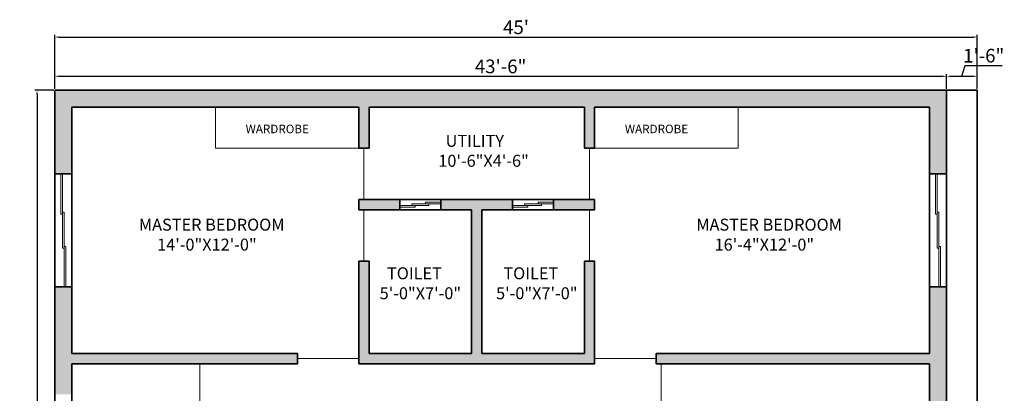
# Model space of a CAD drawing. Units: inches. Extents: x 3491 to 6898, y 1360 to 2019.
# Tile 3 of 9: x 3512 to 4088, y 1795 to 2013. Entities that reach past the tile are written whole.
import ezdxf

# ---------------------------------------------------------------- set-up
doc = ezdxf.new("R2010")
doc.units = ezdxf.units.IN
for name, color, linetype, lineweight in [('A-ANNO-DIMS', 2, 'Continuous', 18), ('A-ANNO-TEXT', 7, 'Continuous', 18), ('A-AREA-IDEN', 7, 'Continuous', 18), ('A-DOOR', 4, 'Continuous', 18), ('A-FLOR-CASE', 8, 'Continuous', 18), ('A-GLAZ', 5, 'Continuous', 18), ('A-WALL', 7, 'Continuous', 35), ('A-WALL-PATT', 8, 'Continuous', 13)]:
    doc.layers.add(name, color=color, linetype=linetype, lineweight=lineweight)
doc.styles.get("Standard").update_dxf_attribs({"font": 'arial.ttf'})
doc.dimstyles.new('ISO-25', dxfattribs={"dimtxt": 8, "dimasz": 2.5, "dimexe": 1.25, "dimexo": 0.625, "dimtad": 1, "dimdec": 1, "dimlunit": 3, "dimtxsty": 'Standard', "dimcen": 2.5, "dimclrt": 1, "dimadec": 0, "dimazin": 0, "dimtfac": 1, "dimtdec": 1, "dimtmove": 0, "dimatfit": 3, "dimfxl": 1, "dimarcsym": 0})

# ---------------------------------------------------------------- blocks, each defined once
blk = doc.blocks.new('*D1')
at = {"layer": 'A-ANNO-DIMS', "color": 0, "lineweight": -2, "transparency": 16777216}
for p, q in [((3532.13, 1972.99), (3532.13, 1981.69)), ((3534.63, 1980.44), (4051.63, 1980.44)), ((4054.13, 1972.99), (4054.13, 1981.69))]:
    blk.add_line(p, q, dxfattribs=at)
at = {"layer": 'A-ANNO-DIMS', "color": 0, "transparency": 16777216}
for points in [[(3534.63, 1980.85), (3534.63, 1980.02), (3532.13, 1980.44)], [(4051.63, 1980.85), (4051.63, 1980.02), (4054.13, 1980.44)]]:
    blk.add_solid(points, dxfattribs=at)
at = {"layer": 'Defpoints', "color": 0, "transparency": 16777216}
for p in [(4054.13, 1980.44), (3532.13, 1972.37), (4054.13, 1972.37)]:
    blk.add_point(p, dxfattribs=at)
at = {"layer": 'A-ANNO-DIMS', "color": 0, "transparency": 16777216, "insert": (3793.13, 1985.15), "char_height": 8, "attachment_point": 5}
blk.add_mtext('43\'-6"', dxfattribs=at)
blk = doc.blocks.new('*D2')
at = {"layer": 'A-ANNO-DIMS', "color": 0, "lineweight": -2, "transparency": 16777216}
for p, q in [((4063.13, 1980.44), (4065.01, 1986.71)), ((4065.01, 1986.71), (4086.78, 1986.71)), ((4054.13, 1972.99), (4054.13, 1981.69)), ((4056.63, 1980.44), (4069.63, 1980.44)), ((4072.13, 1972.99), (4072.13, 1981.69))]:
    blk.add_line(p, q, dxfattribs=at)
at = {"layer": 'A-ANNO-DIMS', "color": 0, "transparency": 16777216}
for points in [[(4056.63, 1980.85), (4056.63, 1980.02), (4054.13, 1980.44)], [(4069.63, 1980.85), (4069.63, 1980.02), (4072.13, 1980.44)]]:
    blk.add_solid(points, dxfattribs=at)
at = {"layer": 'Defpoints', "color": 0, "transparency": 16777216}
for p in [(4072.13, 1980.44), (4054.13, 1972.37), (4072.13, 1972.37)]:
    blk.add_point(p, dxfattribs=at)
at = {"layer": 'A-ANNO-DIMS', "color": 0, "transparency": 16777216, "insert": (4075.9, 1991.42), "char_height": 8, "attachment_point": 5}
blk.add_mtext('1\'-6"', dxfattribs=at)
blk = doc.blocks.new('*D3')
at = {"layer": 'A-ANNO-DIMS', "color": 0, "lineweight": -2, "transparency": 16777216}
for p, q in [((3532.13, 1972.99), (3532.13, 2004.59)), ((3534.63, 2003.34), (4069.63, 2003.34)), ((4072.13, 1972.99), (4072.13, 2004.59))]:
    blk.add_line(p, q, dxfattribs=at)
at = {"layer": 'A-ANNO-DIMS', "color": 0, "transparency": 16777216}
for points in [[(3534.63, 2003.76), (3534.63, 2002.92), (3532.13, 2003.34)], [(4069.63, 2003.76), (4069.63, 2002.92), (4072.13, 2003.34)]]:
    blk.add_solid(points, dxfattribs=at)
at = {"layer": 'Defpoints', "color": 0, "transparency": 16777216}
for p in [(4072.13, 2003.34), (3532.13, 1972.37), (4072.13, 1972.37)]:
    blk.add_point(p, dxfattribs=at)
at = {"layer": 'A-ANNO-DIMS', "color": 0, "transparency": 16777216, "insert": (3802.13, 2008.03), "char_height": 8, "attachment_point": 5}
blk.add_mtext("45'", dxfattribs=at)
blk = doc.blocks.new('*D4')
at = {"layer": 'A-ANNO-DIMS', "color": 0, "lineweight": -2, "transparency": 16777216}
for p, q in [((3531.51, 1972.37), (3520.5, 1972.37)), ((3521.75, 1969.87), (3521.75, 1430.87)), ((3531.51, 1428.37), (3520.5, 1428.37))]:
    blk.add_line(p, q, dxfattribs=at)
at = {"layer": 'A-ANNO-DIMS', "color": 0, "transparency": 16777216}
for points in [[(3521.33, 1969.87), (3522.17, 1969.87), (3521.75, 1972.37)], [(3521.33, 1430.87), (3522.17, 1430.87), (3521.75, 1428.37)]]:
    blk.add_solid(points, dxfattribs=at)
at = {"layer": 'Defpoints', "color": 0, "transparency": 16777216}
for p in [(3532.13, 1972.37), (3521.75, 1428.37), (3532.13, 1428.37)]:
    blk.add_point(p, dxfattribs=at)
at = {"layer": 'A-ANNO-DIMS', "color": 0, "transparency": 16777216, "insert": (3517.06, 1700.37), "char_height": 8, "attachment_point": 5, "rotation": 90}
blk.add_mtext('45\'-4"', dxfattribs=at)
blk = doc.blocks.new('WIN-SLIDER-24IN')
for p, q in [((0, 1), (17, 1)), ((0, 0), (9, 0)), ((7, 1), (7, 2)), ((7, 2), (24, 2)), ((9, 0), (9, 1)), ((15, 2), (15, 3)), ((15, 3), (24, 3)), ((17, 1), (17, 2))]:
    blk.add_line(p, q)
blk = doc.blocks.new('WIN-SLIDER-66IN')
for p, q in [((0, 42.5), (0, 66)), ((1, 22.5), (1, 66)), ((1, 42.5), (0, 42.5)), ((2, 43.5), (1, 43.5)), ((2, 0), (2, 43.5)), ((3, 23.5), (2, 23.5)), ((3, 0), (3, 23.5)), ((2, 22.5), (1, 22.5))]:
    blk.add_line(p, q)

msp = doc.modelspace()

# ---------------------------------------------------------------- hatches: boundary and pattern name
at = {"layer": 'A-WALL-PATT'}
h = msp.add_hatch(color=256, dxfattribs=at)
h.dxf.hatch_style = 1
h.paths.add_polyline_path([(3856.13, 1532.37), (3800.13, 1532.37), (3800.13, 1522.37), (3856.13, 1522.37)])
h.paths.add_polyline_path([(3906.13, 1626.37), (3896.13, 1626.37), (3896.13, 1592.37), (3906.13, 1592.37)])
h.paths.add_polyline_path([(3906.13, 1556.37), (3896.13, 1556.37), (3896.13, 1532.37), (3892.13, 1532.37), (3892.13, 1522.37), (3906.13, 1522.37)])
h.paths.add_polyline_path([(3728.13, 1532.37), (3680.13, 1532.37), (3680.13, 1680.37), (3794.13, 1680.37), (3794.13, 1686.37), (3674.13, 1686.37), (3674.13, 1532.37), (3656.16, 1532.37), (3656.16, 1522.37), (3728.13, 1522.37)])
h.paths.add_polyline_path([(3608.16, 1532.37), (3542.13, 1532.37), (3542.13, 1580.4), (3532.13, 1580.4), (3532.13, 1428.37), (3674.13, 1428.37), (3674.13, 1438.37), (3542.13, 1438.37), (3542.13, 1522.37), (3608.16, 1522.37)])
h.paths.add_polyline_path([(3542.13, 1722.37), (3620.13, 1722.37), (3620.13, 1782.37), (3614.13, 1782.37), (3614.13, 1728.37), (3542.13, 1728.37), (3542.13, 1770.37), (3532.13, 1770.37), (3532.13, 1628.4), (3542.13, 1628.4)])
h.paths.add_polyline_path([(3906.13, 1680.37), (3930.13, 1680.37), (3930.13, 1686.37), (3890.13, 1686.37), (3890.13, 1776.37), (3884.13, 1776.37), (3884.13, 1686.37), (3872.13, 1686.37), (3872.13, 1680.37), (3896.13, 1680.37), (3896.13, 1668.37), (3906.13, 1668.37)])
h.paths.add_polyline_path([(4054.13, 1719.37), (4044.13, 1719.37), (4044.13, 1686.37), (3978.13, 1686.37), (3978.13, 1680.37), (4054.13, 1680.37)])
h.paths.add_polyline_path([(4054.13, 1857.37), (4044.13, 1857.37), (4044.13, 1818.37), (3884.13, 1818.37), (3884.13, 1812.37), (4044.13, 1812.37), (4044.13, 1779.37), (4054.13, 1779.37)])
h.paths.add_polyline_path([(3848.13, 1872.37), (3842.13, 1872.37), (3842.13, 1818.37), (3782.13, 1818.37), (3782.13, 1902.37), (3800.13, 1902.37), (3800.13, 1908.37), (3758.13, 1908.37), (3758.13, 1902.37), (3776.13, 1902.37), (3776.13, 1818.37), (3716.13, 1818.37), (3716.13, 1872.37), (3710.13, 1872.37), (3710.13, 1812.37), (3848.13, 1812.37)])
h.paths.add_polyline_path([(3542.13, 1857.37), (3532.13, 1857.37), (3532.13, 1794.37), (3542.13, 1794.37), (3542.13, 1812.37), (3674.13, 1812.37), (3674.13, 1818.37), (3542.13, 1818.37)])
h.paths.add_polyline_path([(3542.13, 1962.37), (3710.13, 1962.37), (3710.13, 1938.37), (3716.13, 1938.37), (3716.13, 1962.37), (3842.13, 1962.37), (3842.13, 1938.37), (3848.13, 1938.37), (3848.13, 1962.37), (4044.13, 1962.37), (4044.13, 1923.37), (4054.13, 1923.37), (4054.13, 1972.37), (3532.13, 1972.37), (3532.13, 1923.37), (3542.13, 1923.37)])
h.paths.add_polyline_path([(3734.13, 1908.37), (3710.13, 1908.37), (3710.13, 1902.37), (3734.13, 1902.37)])
h.paths.add_polyline_path([(3848.13, 1908.37), (3824.13, 1908.37), (3824.13, 1902.37), (3848.13, 1902.37)], flags=17)

# ---------------------------------------------------------------- linework, layer by layer
at = {"layer": 'A-DOOR'}
for p, q in [((3713.13, 1938.37), (3713.13, 1908.37)), ((3845.13, 1938.37), (3845.13, 1908.37)), ((3713.13, 1872.37), (3713.13, 1902.37)), ((3845.13, 1872.37), (3845.13, 1902.37)), ((3617.13, 1782.37), (3617.13, 1812.37)), ((3674.13, 1815.37), (3710.13, 1815.37)), ((3884.13, 1815.37), (3848.13, 1815.37)), ((3887.13, 1776.37), (3887.13, 1812.37))]:
    msp.add_line(p, q, dxfattribs=at)
at = {"layer": 'A-FLOR-CASE'}
for p, q in [((3626.13, 1962.37), (3626.13, 1938.37)), ((3932.13, 1962.37), (3932.13, 1938.37)), ((3716.13, 1938.37), (3626.13, 1938.37)), ((3932.13, 1938.37), (3842.13, 1938.37))]:
    msp.add_line(p, q, dxfattribs=at)
at = {"layer": 'A-WALL'}
for p, q in [((4072.13, 1972.37), (3532.13, 1972.37)), ((3532.13, 1972.37), (3532.13, 1428.37)), ((4054.13, 1972.37), (4054.13, 1621.37)), ((4072.13, 1428.37), (4072.13, 1972.37)), ((3542.13, 1962.37), (3542.13, 1818.37)), ((3710.13, 1962.37), (3542.13, 1962.37)), ((3710.13, 1962.37), (3710.13, 1938.37)), ((3716.13, 1962.37), (3716.13, 1938.37)), ((3842.13, 1962.37), (3716.13, 1962.37)), ((3842.13, 1962.37), (3842.13, 1938.37)), ((4044.13, 1962.37), (3848.13, 1962.37)), ((3848.13, 1962.37), (3848.13, 1938.37)), ((4044.13, 1962.37), (4044.13, 1818.37)), ((3716.13, 1938.37), (3710.13, 1938.37)), ((3848.13, 1938.37), (3842.13, 1938.37)), ((3542.13, 1923.37), (3532.13, 1923.37)), ((4054.13, 1923.37), (4044.13, 1923.37)), ((3848.13, 1908.37), (3710.13, 1908.37)), ((3710.13, 1908.37), (3710.13, 1902.37)), ((3734.13, 1908.37), (3734.13, 1902.37)), ((3758.13, 1908.37), (3758.13, 1902.37)), ((3800.13, 1908.37), (3800.13, 1902.37)), ((3824.13, 1908.37), (3824.13, 1902.37)), ((3848.13, 1908.37), (3848.13, 1902.37)), ((3776.13, 1902.37), (3710.13, 1902.37)), ((3776.13, 1902.37), (3776.13, 1818.37)), ((3848.13, 1902.37), (3782.13, 1902.37)), ((3782.13, 1902.37), (3782.13, 1818.37)), ((3710.13, 1872.37), (3710.13, 1812.37)), ((3716.13, 1872.37), (3710.13, 1872.37)), ((3716.13, 1872.37), (3716.13, 1818.37)), ((3848.13, 1872.37), (3842.13, 1872.37)), ((3842.13, 1872.37), (3842.13, 1818.37)), ((3848.13, 1872.37), (3848.13, 1812.37)), ((3542.13, 1857.37), (3532.13, 1857.37)), ((4054.13, 1857.37), (4044.13, 1857.37)), ((3674.13, 1818.37), (3542.13, 1818.37)), ((3674.13, 1818.37), (3674.13, 1812.37)), ((3776.13, 1818.37), (3716.13, 1818.37)), ((3842.13, 1818.37), (3782.13, 1818.37)), ((4044.13, 1818.37), (3884.13, 1818.37)), ((3884.13, 1818.37), (3884.13, 1812.37)), ((3542.13, 1812.37), (3542.13, 1728.37)), ((3674.13, 1812.37), (3542.13, 1812.37)), ((3848.13, 1812.37), (3710.13, 1812.37)), ((4044.13, 1812.37), (3884.13, 1812.37)), ((4044.13, 1812.37), (4044.13, 1686.37))]:
    msp.add_line(p, q, dxfattribs=at)

# ---------------------------------------------------------------- block references
at = {"layer": 'A-GLAZ'}
for name, p in [('WIN-SLIDER-66IN', (3535.63, 1857.37)), ('WIN-SLIDER-66IN', (4047.63, 1857.37)), ('WIN-SLIDER-24IN', (3734.13, 1903.87)), ('WIN-SLIDER-24IN', (3800.13, 1903.87))]:
    msp.add_blockref(name, p, dxfattribs=at)

# ---------------------------------------------------------------- texts
at = {"layer": 'A-ANNO-TEXT', "char_height": 5, "attachment_point": 1}
for insert in [(3643.84, 1952.13), (3865.84, 1952.13)]:
    msp.add_mtext_dynamic_manual_height_columns('WARDROBE', width=86.9528, gutter_width=12.5, heights=[0], dxfattribs=dict(at, insert=insert))
at = {"layer": 'A-AREA-IDEN', "char_height": 7, "attachment_point": 1}
for s, insert in [('  UTILITY\\P10\'-6"X4\'-6"', (3756.64, 1946.16)), ('MASTER BEDROOM\\P     14\'-0"X12\'-0"', (3581.37, 1897.15)), ('MASTER BEDROOM\\P     16\'-4"X12\'-0"', (3907.66, 1897.15)), ('  TOILET\\P5\'-0"X7\'-0"', (3722.32, 1868.72)), ('  TOILET\\P5\'-0"X7\'-0"', (3790.46, 1868.72))]:
    msp.add_mtext_dynamic_manual_height_columns(s, width=121.6144, gutter_width=12.5, heights=[0], dxfattribs=dict(at, insert=insert))

# ---------------------------------------------------------------- dimensions: what is measured, and where the dimension line sits
at = {"layer": 'A-ANNO-DIMS'}
for base, p1, p2, override, picture, middle in [((4072.13, 2003.34), (3532.13, 1972.37), (4072.13, 1972.37), {"dimclrd": 0, "dimclre": 0, "dimclrt": 0}, '*D3', (3802.13, 2008.03)), ((4072.13, 1980.44), (4054.13, 1972.37), (4072.13, 1972.37), {"dimclrd": 0, "dimclre": 0, "dimclrt": 0, "dimtmove": 1}, '*D2', (4065.64, 1991.42)), ((4054.13, 1980.44), (3532.13, 1972.37), (4054.13, 1972.37), {"dimclrd": 0, "dimclre": 0, "dimclrt": 0}, '*D1', (3793.13, 1985.15))]:
    dim = msp.add_linear_dim(base=base, p1=p1, p2=p2, dimstyle='ISO-25', override=override, dxfattribs=at)
    dim.commit()
    dim.dimension.update_dxf_attribs({"geometry": picture, "text_midpoint": middle})
dim = msp.add_linear_dim(base=(3521.75, 1428.37), p1=(3532.13, 1972.37), p2=(3532.13, 1428.37), angle=90, dimstyle='ISO-25', override={"dimclrd": 0, "dimclre": 0, "dimclrt": 0}, dxfattribs=at)
dim.commit()
dim.dimension.update_dxf_attribs({"geometry": '*D4', "text_midpoint": (3517.06, 1700.37)})

doc.saveas('drawing.dxf')
